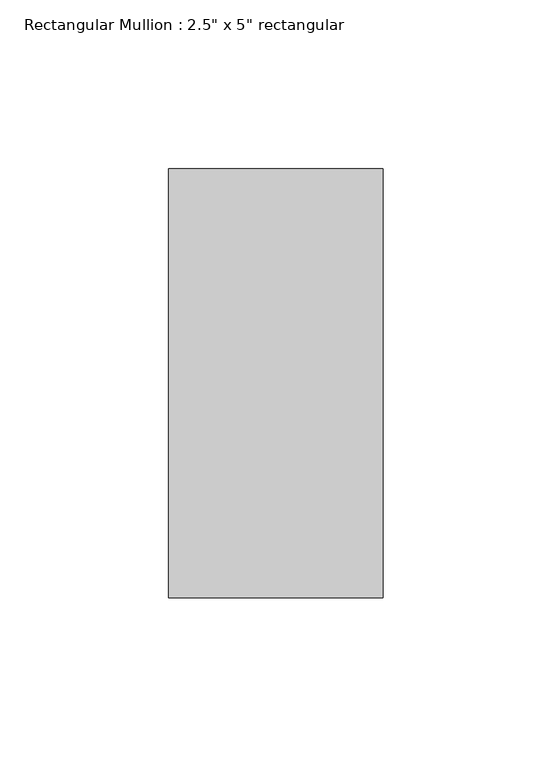
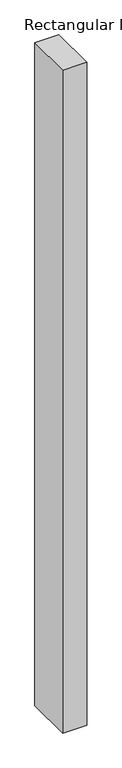
"""IFC4 building model written with IfcOpenShell, lengths in millimetres: member geometry."""

from ifc_helpers import new_model, si_unit, frame, origin, place, context, project, spatial, polyline, outline, extrude, source, transform, mapped, element, save


def member_d73967ec(model_context):
    return source(origin(), model_context, "Body", "SweptSolid", [
        extrude(outline(polyline([(31.75, 63.5), (31.75, -63.5), (-31.75, -63.5), (-31.75, 63.5), (31.75, 63.5)])), frame((0.0, 0.0, -1854.2), z_axis=(0.0, 0.0, 1.0), x_axis=(1.0, 0.0, 0.0)), (0.0, 0.0, 1.0), 1854.2),
    ])


if __name__ == "__main__":
    model = new_model("IFC4")
    model_context = context("Model", 3, world=origin())
    ifc_project = project(units=[si_unit("LENGTHUNIT", "METRE", prefix="MILLI")], contexts=[model_context])
    site = spatial("IfcSite", under=ifc_project)
    building = spatial("IfcBuilding", under=site)
    placement = place(None, origin())
    member_shape = member_d73967ec(model_context)
    element("IfcMember", 1, ObjectType="Rectangular Mullion : 2.5\" x 5\" rectangular", at=placement, inside=building, context=model_context, shape_type="MappedRepresentation", body=[
        mapped(member_shape, transform((0.0, 0.0, 0.0), x_axis=(1.0, 0.0, 0.0), y_axis=(0.0, 1.0, 0.0), z_axis=(0.0, 0.0, 1.0))),
    ])
    save(model, "model.ifc")

# Revit data of these elements
# Type "Rectangular Mullion : 2.5\" x 5\" rectangular"
#   built-in parameter 1007304 = 0.416667 (stored number, unit not read)
#   built-in parameter 1007301 = 0.104167 (stored number, unit not read)
#   built-in parameter 1007300 = 0.104167 (stored number, unit not read)
# Element 1 (IfcMember, "Rectangular Mullion : 2.5\" x 5\" rectangular")
#   Materials on its faces: "Aluminum"
# Materials
#   "Aluminum": class "Metal", colour RGB 247 247 247, transparency 0, Description = "Aluminum 6061", Cost = 0
